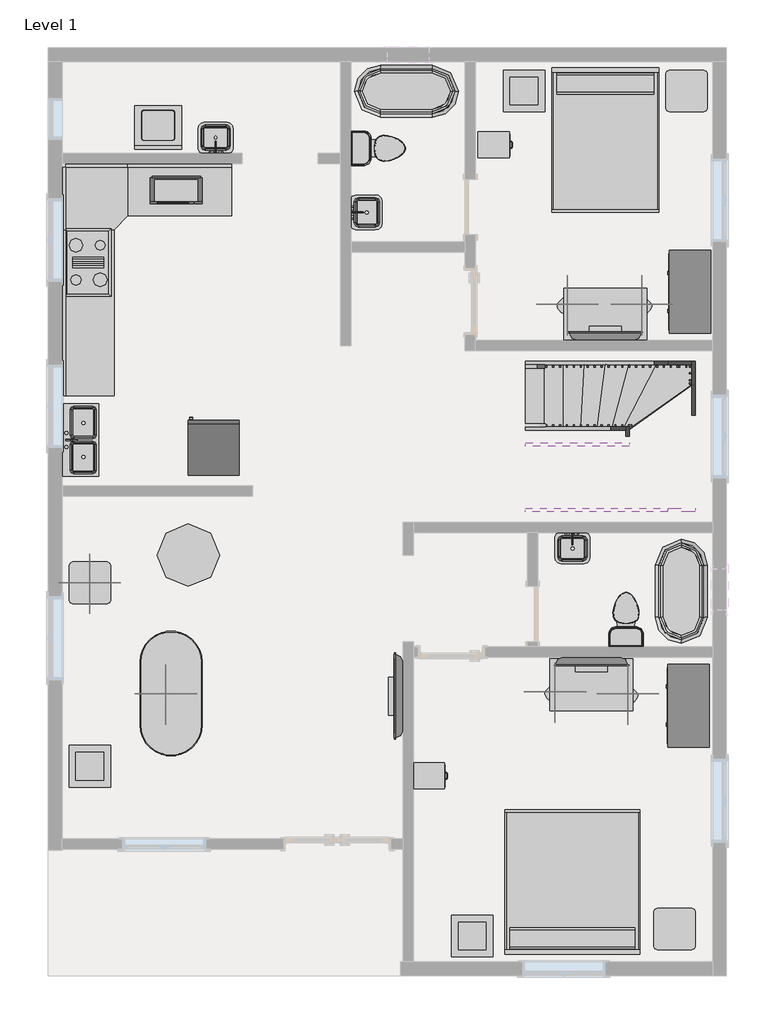
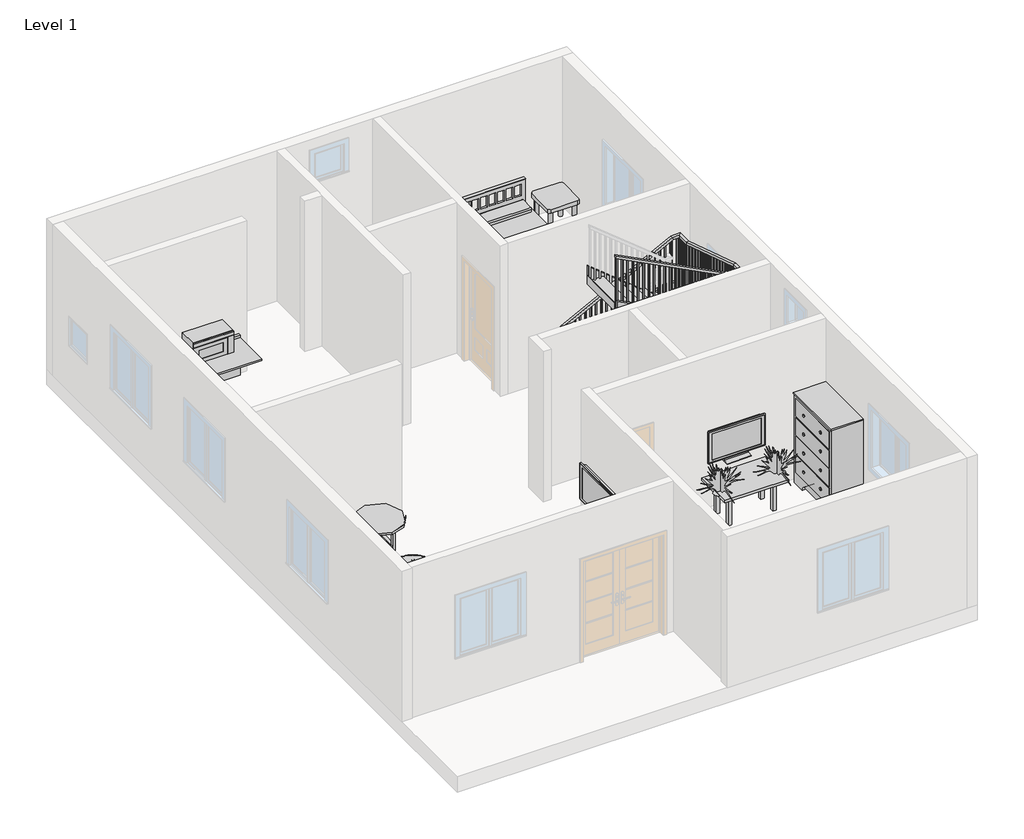
# One storey, part 2 of 2: 20 furniture elements, 11 flow terminals, 8 members, 6 geographic elements, 4 proxies, 1 railing, 1 stair flight.
"""IFC4 building model written with IfcOpenShell, lengths in millimetres."""

from ifc_helpers import new_model, si_unit, frame, origin, place, context, project, spatial, polyline, outline, extrude, faceted_brep, transform, mapped, element, save
from components import proxy_bb1e6e30, proxy_8a8d5ab2, proxy_a13a33b2, proxy_718fa39f, flow_terminal_accce45a, flow_terminal_a53be723, flow_terminal_62a433f7, toilet_domestic_3d_toilet_domestic_3d_f7549cf7, toilet_domestic_3d_toilet_domestic_3d_183bbd19, flow_terminal_b374fae2, furniture_29cd36cd, furniture_35c09872, furniture_bb55ed6b, furniture_9fa109b2, furniture_7a3aaa4f, furniture_fdf74506, furniture_b5c51a22, furniture_2c34a4f9, furniture_905aceb5, furniture_31d08a24, furniture_3f969c1c, furniture_f7403a93, rpc_plant_tropical_agave_1_5_93a2a214, stair_flight_cbf97d32

model = new_model("IFC4")

# Units and contexts
model_context = context("Model", 3, world=origin())
ifc_project = project(units=[si_unit("LENGTHUNIT", "METRE", prefix="MILLI")], contexts=[model_context])

# Site, building, storey
site = spatial("IfcSite", under=ifc_project)
building = spatial("IfcBuilding", under=site)
storey = spatial("IfcBuildingStorey", under=building, Name="Level 1", Elevation=0.0)

# Proxies
placement = place(None, origin())
proxy_shape = proxy_bb1e6e30(model_context)
element("IfcBuildingElementProxy", 1, Name="Cook Top-4 Unit : 36\" x 20\"", ObjectType="Cook Top-4 Unit : 36\" x 20\"", at=placement, inside=storey, context=model_context, shape_type="MappedRepresentation", body=[
    mapped(proxy_shape, transform((-14225.9837964, 8614.5759458, 0.0), x_axis=(0.0, 1.0, 0.0), y_axis=(-1.0, 0.0, 0.0), z_axis=(0.0, 0.0, 1.0))),
])
proxy_2_shape = proxy_8a8d5ab2(model_context)
element("IfcBuildingElementProxy", 2, Name="Microwave : 30\" x 16\" x 18\"", ObjectType="Microwave : 30\" x 16\" x 18\"", at=placement, inside=storey, context=model_context, shape_type="MappedRepresentation", body=[
    mapped(proxy_2_shape, transform((-13430.8766737, 10034.4564516, 0.0), x_axis=(1.0000000000000009, 0.0, 0.0), y_axis=(0.0, 1.0000000000000009, 0.0), z_axis=(0.0, 0.0, 1.0))),
])
proxy_3_shape = proxy_a13a33b2(model_context)
element("IfcBuildingElementProxy", 3, Name="Refrigerator : 30\" x 32\" RH", ObjectType="Refrigerator : 30\" x 32\" RH", at=placement, inside=storey, context=model_context, shape_type="MappedRepresentation", body=[
    mapped(proxy_3_shape, transform((-12379.7212964, 5878.9249173, 0.0), x_axis=(-1.0000000000000004, 0.0, 0.0), y_axis=(0.0, -1.0000000000000004, 0.0), z_axis=(0.0, 0.0, 1.0))),
])
proxy_4_shape = proxy_718fa39f(model_context)
element("IfcBuildingElementProxy", 4, Name="Washer : 27\" x 25\" x 35\"", ObjectType="Washer : 27\" x 25\" x 35\"", at=placement, inside=storey, context=model_context, shape_type="MappedRepresentation", body=[
    mapped(proxy_4_shape, transform((-12776.8663279, 10874.9255106, 0.0), x_axis=(-1.0000000000000004, 0.0, 0.0), y_axis=(0.0, -1.0000000000000004, 0.0), z_axis=(0.0, 0.0, 1.0))),
])

# Flow terminals
flow_terminal_shape = flow_terminal_accce45a(model_context)
element("IfcFlowTerminal", 5, ObjectType="Floor Drain - Round : 5\" Strainer - 2\" Drain", at=placement, inside=storey, context=model_context, shape_type="MappedRepresentation", body=[
    mapped(flow_terminal_shape, transform((-12574.9837964, 11357.7759458, 0.0), x_axis=(1.0, 0.0, 0.0), y_axis=(0.0, 1.0, 0.0), z_axis=(0.0, 0.0, 1.0))),
])
element("IfcFlowTerminal", 6, ObjectType="Floor Drain - Round : 5\" Strainer - 2\" Drain", at=placement, inside=storey, context=model_context, shape_type="MappedRepresentation", body=[
    mapped(flow_terminal_shape, transform((-8841.1837964, 10494.1759458, 0.0), x_axis=(1.0, 0.0, 0.0), y_axis=(0.0, 1.0, 0.0), z_axis=(0.0, 0.0, 1.0))),
])
element("IfcFlowTerminal", 7, ObjectType="Floor Drain - Round : 5\" Strainer - 2\" Drain", at=placement, inside=storey, context=model_context, shape_type="MappedRepresentation", body=[
    mapped(flow_terminal_shape, transform((-6148.7837964, 4372.7759458, 0.0), x_axis=(1.0, 0.0, 0.0), y_axis=(0.0, 1.0, 0.0), z_axis=(0.0, 0.0, 1.0))),
])
flow_terminal_2_shape = flow_terminal_a53be723(model_context)
element("IfcFlowTerminal", 8, ObjectType="Sink Kitchen-Double : 42\" x 21\"", at=placement, inside=storey, context=model_context, shape_type="MappedRepresentation", body=[
    mapped(flow_terminal_2_shape, transform((-14331.5883953, 5995.3867052, 0.0), x_axis=(0.0, 1.0000000000000002, 0.0), y_axis=(-1.0000000000000002, 0.0, 0.0), z_axis=(0.0, 0.0, 1.0))),
])
flow_terminal_3_shape = flow_terminal_62a433f7(model_context)
element("IfcFlowTerminal", 9, ObjectType="Sink Vanity-Square : 20\" x 18\"", at=placement, inside=storey, context=model_context, shape_type="MappedRepresentation", body=[
    mapped(flow_terminal_3_shape, transform((-12337.0445558, 10394.9213469, 0.0), x_axis=(-1.0000000000000002, 0.0, 0.0), y_axis=(0.0, -1.0000000000000002, 0.0), z_axis=(0.0, 0.0, 1.0))),
])
element("IfcFlowTerminal", 10, ObjectType="Sink Vanity-Square : 20\" x 18\"", at=placement, inside=storey, context=model_context, shape_type="MappedRepresentation", body=[
    mapped(flow_terminal_3_shape, transform((-10185.0383953, 9335.4867052, 0.0), x_axis=(0.0, 1.0000000000000002, 0.0), y_axis=(-1.0000000000000002, 0.0, 0.0), z_axis=(0.0, 0.0, 1.0))),
])
element("IfcFlowTerminal", 11, ObjectType="Sink Vanity-Square : 20\" x 18\"", at=placement, inside=storey, context=model_context, shape_type="MappedRepresentation", body=[
    mapped(flow_terminal_3_shape, transform((-7129.6730369, 4472.0305447, 0.0), x_axis=(1.0, 0.0, 0.0), y_axis=(0.0, 1.0, 0.0), z_axis=(0.0, 0.0, 1.0))),
])
toilet_domestic_3d_toilet_domestic_3d_shape = toilet_domestic_3d_toilet_domestic_3d_f7549cf7(model_context)
toilet_domestic_3d_toilet_domestic_3d_2_shape = toilet_domestic_3d_toilet_domestic_3d_183bbd19(model_context)
element("IfcFlowTerminal", 12, ObjectType="Toilet-Domestic-3D : Toilet-Domestic-3D", at=placement, inside=storey, context=model_context, shape_type="MappedRepresentation", body=[
    mapped(toilet_domestic_3d_toilet_domestic_3d_shape, transform((-9870.487769, 10290.9759458, 0.0), x_axis=(0.0, 1.0000000000000002, 0.0), y_axis=(-1.0000000000000002, 0.0, 0.0), z_axis=(0.0, 0.0, 1.0))),
    mapped(toilet_domestic_3d_toilet_domestic_3d_2_shape, transform((-9870.487769, 10290.9759458, 0.0), x_axis=(0.0, 1.0000000000000002, 0.0), y_axis=(-1.0000000000000002, 0.0, 0.0), z_axis=(0.0, 0.0, 1.0))),
])
element("IfcFlowTerminal", 13, ObjectType="Toilet-Domestic-3D : Toilet-Domestic-3D", at=placement, inside=storey, context=model_context, shape_type="MappedRepresentation", body=[
    mapped(toilet_domestic_3d_toilet_domestic_3d_shape, transform((-6326.5837964, 3470.4719732, 0.0), x_axis=(-1.0000000000000004, 0.0, 0.0), y_axis=(0.0, -1.0000000000000004, 0.0), z_axis=(0.0, 0.0, 1.0))),
    mapped(toilet_domestic_3d_toilet_domestic_3d_2_shape, transform((-6326.5837964, 3470.4719732, 0.0), x_axis=(-1.0000000000000004, 0.0, 0.0), y_axis=(0.0, -1.0000000000000004, 0.0), z_axis=(0.0, 0.0, 1.0))),
])
flow_terminal_4_shape = flow_terminal_b374fae2(model_context)
element("IfcFlowTerminal", 14, ObjectType="Tub-Free Standing-3D : 30\" x 60\"", at=placement, inside=storey, context=model_context, shape_type="MappedRepresentation", body=[
    mapped(flow_terminal_4_shape, transform((-9552.3837964, 11129.1759458, 0.0), x_axis=(0.0, 1.0000000000000002, 0.0), y_axis=(-1.0000000000000002, 0.0, 0.0), z_axis=(0.0, 0.0, 1.0))),
])
element("IfcFlowTerminal", 15, ObjectType="Tub-Free Standing-3D : 30\" x 60\"", at=placement, inside=storey, context=model_context, shape_type="MappedRepresentation", body=[
    mapped(flow_terminal_4_shape, transform((-5513.7837964, 3788.5759458, 0.0), x_axis=(1.0, 0.0, 0.0), y_axis=(0.0, 1.0, 0.0), z_axis=(0.0, 0.0, 1.0))),
])

# Furniture
furniture_shape = furniture_29cd36cd(model_context)
element("IfcFurniture", 16, ObjectType="Bed-Shaker : King 78\" x 83\"", at=placement, inside=storey, context=model_context, shape_type="MappedRepresentation", body=[
    mapped(furniture_shape, transform((-7133.0337964, -1520.0240542, 0.0), x_axis=(-1.0000000000000002, 0.0, 0.0), y_axis=(0.0, -1.0000000000000002, 0.0), z_axis=(0.0, 0.0, 1.0))),
])
furniture_2_shape = furniture_35c09872(model_context)
element("IfcFurniture", 17, ObjectType="Bed-Shaker : Queen 62\" x 83\"", at=placement, inside=storey, context=model_context, shape_type="MappedRepresentation", body=[
    mapped(furniture_2_shape, transform((-6612.3337964, 11459.3759458, 0.0), x_axis=(1.0, 0.0, 0.0), y_axis=(0.0, 1.0, 0.0), z_axis=(0.0, 0.0, 1.0))),
])
furniture_3_shape = furniture_bb55ed6b(model_context)
element("IfcFurniture", 18, ObjectType="Cabinet-File 2 Drawer : 15\" x 18\"", at=placement, inside=storey, context=model_context, shape_type="MappedRepresentation", body=[
    mapped(furniture_3_shape, transform((-8411.8180965, 10469.6723928, 0.0), x_axis=(0.0, 1.0000000000000002, 0.0), y_axis=(-1.0000000000000002, 0.0, 0.0), z_axis=(0.0, 0.0, 1.0))),
])
element("IfcFurniture", 19, ObjectType="Cabinet-File 2 Drawer : 15\" x 18\"", at=placement, inside=storey, context=model_context, shape_type="MappedRepresentation", body=[
    mapped(furniture_3_shape, transform((-9364.3180965, 1211.3723928, 0.0), x_axis=(0.0, 1.0, 0.0), y_axis=(-1.0, 0.0, 0.0), z_axis=(0.0, 0.0, 1.0))),
])
furniture_4_shape = furniture_9fa109b2(model_context)
element("IfcFurniture", 20, ObjectType="Dresser : 48\" x 72\" x 24\"", at=placement, inside=storey, context=model_context, shape_type="MappedRepresentation", body=[
    mapped(furniture_4_shape, transform((-5023.6208423, 7913.582686, 0.0), x_axis=(0.0, -1.0000000000000007, 0.0), y_axis=(1.0000000000000007, 0.0, 0.0), z_axis=(0.0, 0.0, 1.0))),
])
element("IfcFurniture", 21, ObjectType="Dresser : 48\" x 72\" x 24\"", at=placement, inside=storey, context=model_context, shape_type="MappedRepresentation", body=[
    mapped(furniture_4_shape, transform((-5049.0208423, 1842.982686, 0.0), x_axis=(0.0, -1.0000000000000004, 0.0), y_axis=(1.0000000000000004, 0.0, 0.0), z_axis=(0.0, 0.0, 1.0))),
])
furniture_5_shape = furniture_7a3aaa4f(model_context)
element("IfcFurniture", 22, ObjectType="TV - Flat Screen : 42\"", at=placement, inside=storey, context=model_context, shape_type="MappedRepresentation", body=[
    mapped(furniture_5_shape, transform((-6635.3283105, 7530.1145695, 914.4), x_axis=(-1.0000000000000004, 0.0, 0.0), y_axis=(0.0, -1.0000000000000004, 0.0), z_axis=(0.0, 0.0, 1.0))),
])
element("IfcFurniture", 23, ObjectType="TV - Flat Screen : 42\"", at=placement, inside=storey, context=model_context, shape_type="MappedRepresentation", body=[
    mapped(furniture_5_shape, transform((-6830.6392822, 2764.8373222, 914.4), x_axis=(1.0, 0.0, 0.0), y_axis=(0.0, 1.0, 0.0), z_axis=(0.0, 0.0, 1.0))),
])
furniture_6_shape = furniture_fdf74506(model_context)
element("IfcFurniture", 24, ObjectType="TV - Flat Screen : 50\"", at=placement, inside=storey, context=model_context, shape_type="MappedRepresentation", body=[
    mapped(furniture_6_shape, transform((-9661.72242, 2247.9314317, 914.4), x_axis=(0.0, -1.0000000000000002, 0.0), y_axis=(1.0000000000000002, 0.0, 0.0), z_axis=(0.0, 0.0, 1.0))),
])
furniture_7_shape = furniture_b5c51a22(model_context)
element("IfcFurniture", 25, ObjectType="Table-Coffee : 24\" x 24\" x 24\"", at=placement, inside=storey, context=model_context, shape_type="MappedRepresentation", body=[
    mapped(furniture_7_shape, transform((-7843.449563, 11033.964868, 0.0), x_axis=(1.0, 0.0, 0.0), y_axis=(0.0, 1.0, 0.0), z_axis=(0.0, 0.0, 1.0))),
])
element("IfcFurniture", 26, ObjectType="Table-Coffee : 24\" x 24\" x 24\"", at=placement, inside=storey, context=model_context, shape_type="MappedRepresentation", body=[
    mapped(furniture_7_shape, transform((-8605.449563, -1361.235132, 0.0), x_axis=(1.0, 0.0, 0.0), y_axis=(0.0, 1.0, 0.0), z_axis=(0.0, 0.0, 1.0))),
])
element("IfcFurniture", 27, ObjectType="Table-Coffee : 24\" x 24\" x 24\"", at=placement, inside=storey, context=model_context, shape_type="MappedRepresentation", body=[
    mapped(furniture_7_shape, transform((-14218.849563, 1127.964868, 0.0), x_axis=(1.0, 0.0, 0.0), y_axis=(0.0, 1.0, 0.0), z_axis=(0.0, 0.0, 1.0))),
])
furniture_8_shape = furniture_2c34a4f9(model_context)
element("IfcFurniture", 28, ObjectType="Table-Dining Oval : 36\" x 72\"", at=placement, inside=storey, context=model_context, shape_type="MappedRepresentation", body=[
    mapped(furniture_8_shape, transform((-13364.882157, 2691.7956179, 0.0), x_axis=(0.0, 1.0, 0.0), y_axis=(-1.0, 0.0, 0.0), z_axis=(0.0, 0.0, 1.0))),
])
furniture_9_shape = furniture_905aceb5(model_context)
element("IfcFurniture", 29, ObjectType="Table-Dining Round w Chairs : 36\" Diameter", at=placement, inside=storey, context=model_context, shape_type="MappedRepresentation", body=[
    mapped(furniture_9_shape, transform((-12856.4657636, 4506.8546343, 0.0), x_axis=(1.0, 0.0, 0.0), y_axis=(0.0, 1.0, 0.0), z_axis=(0.0, 0.0, 1.0))),
])
furniture_10_shape = furniture_31d08a24(model_context)
element("IfcFurniture", 30, ObjectType="Table-End : 24\" x 24\"", at=placement, inside=storey, context=model_context, shape_type="MappedRepresentation", body=[
    mapped(furniture_10_shape, transform((-5746.1174267, 10976.7759458, 0.0), x_axis=(1.0, 0.0, 0.0), y_axis=(0.0, 1.0, 0.0), z_axis=(0.0, 0.0, 1.0))),
])
element("IfcFurniture", 31, ObjectType="Table-End : 24\" x 24\"", at=placement, inside=storey, context=model_context, shape_type="MappedRepresentation", body=[
    mapped(furniture_10_shape, transform((-5923.9174267, -1316.8240542, 0.0), x_axis=(1.0, 0.0, 0.0), y_axis=(0.0, 1.0, 0.0), z_axis=(0.0, 0.0, 1.0))),
])
element("IfcFurniture", 32, ObjectType="Table-End : 24\" x 24\"", at=placement, inside=storey, context=model_context, shape_type="MappedRepresentation", body=[
    mapped(furniture_10_shape, transform((-14509.1174267, 3763.1759458, 0.0), x_axis=(1.0, 0.0, 0.0), y_axis=(0.0, 1.0, 0.0), z_axis=(0.0, 0.0, 1.0))),
])
furniture_11_shape = furniture_3f969c1c(model_context)
element("IfcFurniture", 33, ObjectType="Table-Rectangular : 72\" x 30\"", at=placement, inside=storey, context=model_context, shape_type="MappedRepresentation", body=[
    mapped(furniture_11_shape, transform((-6834.5837964, 2416.9759458, 0.0), x_axis=(1.0, 0.0, 0.0), y_axis=(0.0, 1.0, 0.0), z_axis=(0.0, 0.0, 1.0))),
])
element("IfcFurniture", 34, ObjectType="Table-Rectangular : 72\" x 30\"", at=placement, inside=storey, context=model_context, shape_type="MappedRepresentation", body=[
    mapped(furniture_11_shape, transform((-6631.3837964, 7852.5759458, 0.0), x_axis=(1.0, 0.0, 0.0), y_axis=(0.0, 1.0, 0.0), z_axis=(0.0, 0.0, 1.0))),
])
furniture_12_shape = furniture_f7403a93(model_context)
element("IfcFurniture", 35, ObjectType="Work Station Cubicle : 96\" x 96\"", at=placement, inside=storey, context=model_context, shape_type="MappedRepresentation", body=[
    mapped(furniture_12_shape, transform((-14475.2520442, 10557.3989534, 0.0), x_axis=(1.0, 0.0, 0.0), y_axis=(0.0, 1.0, 0.0), z_axis=(0.0, 0.0, 1.0))),
])

# Geographic elements
rpc_plant_tropical_agave_1_5_shape = rpc_plant_tropical_agave_1_5_93a2a214(model_context)
element("IfcGeographicElement", 36, ObjectType="RPC Plant - Tropical : Agave - 1.5'", at=placement, inside=storey, context=model_context, shape_type="MappedRepresentation", body=[
    mapped(rpc_plant_tropical_agave_1_5_shape, transform((-14200.5837964, 3915.5759458, 609.6), x_axis=(1.0, 0.0, 0.0), y_axis=(0.0, 1.0, 0.0), z_axis=(0.0, 0.0, 1.0))),
])
element("IfcGeographicElement", 37, ObjectType="RPC Plant - Tropical : Agave - 1.5'", at=placement, inside=storey, context=model_context, shape_type="MappedRepresentation", body=[
    mapped(rpc_plant_tropical_agave_1_5_shape, transform((-13082.9837964, 2289.9759458, 736.6), x_axis=(1.0, 0.0, 0.0), y_axis=(0.0, 1.0, 0.0), z_axis=(0.0, 0.0, 1.0))),
])
element("IfcGeographicElement", 38, ObjectType="RPC Plant - Tropical : Agave - 1.5'", at=placement, inside=storey, context=model_context, shape_type="MappedRepresentation", body=[
    mapped(rpc_plant_tropical_agave_1_5_shape, transform((-7367.9837964, 2315.3759458, 660.4), x_axis=(1.0, 0.0, 0.0), y_axis=(0.0, 1.0, 0.0), z_axis=(0.0, 0.0, 1.0))),
])
element("IfcGeographicElement", 39, ObjectType="RPC Plant - Tropical : Agave - 1.5'", at=placement, inside=storey, context=model_context, shape_type="MappedRepresentation", body=[
    mapped(rpc_plant_tropical_agave_1_5_shape, transform((-6301.1837964, 2289.9759458, 660.4), x_axis=(1.0, 0.0, 0.0), y_axis=(0.0, 1.0, 0.0), z_axis=(0.0, 0.0, 1.0))),
])
element("IfcGeographicElement", 40, ObjectType="RPC Plant - Tropical : Agave - 1.5'", at=placement, inside=storey, context=model_context, shape_type="MappedRepresentation", body=[
    mapped(rpc_plant_tropical_agave_1_5_shape, transform((-7190.1837964, 8004.9759458, 660.4), x_axis=(1.0, 0.0, 0.0), y_axis=(0.0, 1.0, 0.0), z_axis=(0.0, 0.0, 1.0))),
])
element("IfcGeographicElement", 41, ObjectType="RPC Plant - Tropical : Agave - 1.5'", at=placement, inside=storey, context=model_context, shape_type="MappedRepresentation", body=[
    mapped(rpc_plant_tropical_agave_1_5_shape, transform((-6097.9837964, 8004.9759458, 660.4), x_axis=(1.0, 0.0, 0.0), y_axis=(0.0, 1.0, 0.0), z_axis=(0.0, 0.0, 1.0))),
])

# Members
element("IfcMember", 42, ObjectType="Stringer - 2\" Width", at=placement, inside=storey, context=model_context, shape_type="SweptSolid", body=[
    extrude(outline(polyline([(229.639954, -7803.5154882), (0.0, -7803.5154882), (0.0, -7583.7531707), (962.500629, -5716.0982966), (1305.3956453, -5716.0982966), (229.639954, -7803.5154882)])), frame((0.0, 7115.9759458, 0.0), z_axis=(0.0, 1.0, 0.0), x_axis=(0.0, 0.0, 1.0)), (0.0, 0.0, 1.0), 50.8),
])
element("IfcMember", 43, ObjectType="Stringer - 2\" Width", at=placement, inside=storey, context=model_context, shape_type="SweptSolid", body=[
    extrude(outline(polyline([(-5716.0982966, 7115.9759458), (-5716.0982966, 7166.7759458), (-5361.3837964, 7166.7759458), (-5361.3837964, 7115.9759458), (-5716.0982966, 7115.9759458)])), frame((0.0, 0.0, 962.500629), z_axis=(0.0, 0.0, 1.0), x_axis=(1.0, 0.0, 0.0)), (0.0, 0.0, 1.0), 342.8950162),
])
element("IfcMember", 44, ObjectType="Stringer - 2\" Width", at=placement, inside=storey, context=model_context, shape_type="SweptSolid", body=[
    extrude(outline(polyline([(7166.7759458, 1289.0952212), (7166.7759458, 1000.5956453), (6997.2534628, 1000.5956453), (5007.7759458, 1638.9682298), (5007.7759458, 1969.9972697), (5044.7560631, 1969.9972697), (7166.7759458, 1289.0952212)])), frame((-5361.3837964, 0.0, 0.0), z_axis=(1.0, 0.0, 0.0), x_axis=(0.0, 1.0, 0.0)), (0.0, 0.0, 1.0), 50.8),
])
element("IfcMember", 45, ObjectType="Stringer - 2\" Width", at=placement, inside=storey, context=model_context, shape_type="SweptSolid", body=[
    extrude(outline(polyline([(-5310.5837964, 5007.7759458), (-5310.5837964, 4956.9759458), (-5716.0982966, 4956.9759458), (-5716.0982966, 5007.7759458), (-5310.5837964, 5007.7759458)])), frame((0.0, 0.0, 1649.8904473), z_axis=(0.0, 0.0, 1.0), x_axis=(1.0, 0.0, 0.0)), (0.0, 0.0, 1.0), 320.1068224),
])
element("IfcMember", 46, ObjectType="Stringer - 2\" Width", at=placement, inside=storey, context=model_context, shape_type="SweptSolid", body=[
    extrude(outline(polyline([(1649.8904473, -5716.0982966), (1969.9972697, -5716.0982966), (3045.7529609, -7803.5154882), (2725.6461385, -7803.5154882), (1649.8904473, -5716.0982966)])), frame((0.0, 4956.9759458, 0.0), z_axis=(0.0, 1.0, 0.0), x_axis=(0.0, 0.0, 1.0)), (0.0, 0.0, 1.0), 50.8),
])
element("IfcMember", 47, ObjectType="Stringer - 2\" Width", at=placement, inside=storey, context=model_context, shape_type="SweptSolid", body=[
    extrude(outline(polyline([(176.1764461, -7803.5154882), (0.0, -7803.5154882), (0.0, -7537.2538437), (987.1410923, -6326.5837964), (1380.418648, -6326.5837964), (176.1764461, -7803.5154882)])), frame((0.0, 6150.7759458, 0.0), z_axis=(0.0, 1.0, 0.0), x_axis=(0.0, 0.0, 1.0)), (0.0, 0.0, 1.0), 50.8),
])
element("IfcMember", 48, ObjectType="Stringer - 2\" Width", at=placement, inside=storey, context=model_context, shape_type="SweptSolid", body=[
    extrude(outline(polyline([(6201.5759458, 1573.2682978), (6201.5759458, 1028.5617647), (6167.3337285, 1028.5617647), (5972.9759458, 1360.465107), (5972.9759458, 1926.1409689), (5994.9388284, 1926.1409689), (6201.5759458, 1573.2682978)])), frame((-6326.5837964, 0.0, 0.0), z_axis=(1.0, 0.0, 0.0), x_axis=(0.0, 1.0, 0.0)), (0.0, 0.0, 1.0), 50.8),
])
element("IfcMember", 49, ObjectType="Stringer - 2\" Width", at=placement, inside=storey, context=model_context, shape_type="SweptSolid", body=[
    extrude(outline(polyline([(1532.8634131, -6275.7837964), (1926.1409689, -6275.7837964), (3171.8038432, -7803.5154882), (2778.5262875, -7803.5154882), (1532.8634131, -6275.7837964)])), frame((0.0, 5922.1759458, 0.0), z_axis=(0.0, 1.0, 0.0), x_axis=(0.0, 0.0, 1.0)), (0.0, 0.0, 1.0), 50.8),
])

# Railing
element("IfcRailing", 50, ObjectType="Handrail - Rectangular", at=placement, inside=storey, context=model_context, shape_type="SolidModel", body=[
    faceted_brep([(-7803.5154882, 7115.9759458, 1109.0771751), (-7803.5154882, 7115.9759458, 1051.9280057), (-7803.5154882, 7065.1759458, 1051.9280057), (-7803.5154882, 7065.1759458, 1109.0771751), (-5543.5336317, 7115.9759458, 2273.7644996), (-5531.2135805, 7115.9759458, 2222.9644996), (-5531.2135805, 7065.1759458, 2222.9644996), (-5543.5336317, 7065.1759458, 2273.7644996), (-5361.3837964, 7115.9759458, 2273.7644996), (-5361.3837964, 7115.9759458, 2222.9644996), (-5412.1837964, 7065.1759458, 2222.9644996), (-5412.1837964, 7065.1759458, 2273.7644996), (-5361.3837964, 6838.8219932, 2273.7644996), (-5361.3837964, 6830.8714171, 2222.9644996), (-5412.1837964, 6830.8714171, 2222.9644996), (-5412.1837964, 6838.8219932, 2273.7644996), (-5361.3837964, 5284.9298984, 2772.3688337), (-5361.3837964, 5276.9793223, 2721.5688337), (-5412.1837964, 5276.9793223, 2721.5688337), (-5412.1837964, 5284.9298984, 2772.3688337), (-5361.3837964, 5007.7759458, 2772.3688337), (-5361.3837964, 5007.7759458, 2721.5688337), (-5412.1837964, 5058.5759458, 2721.5688337), (-5412.1837964, 5058.5759458, 2772.3688337), (-5543.5336317, 5007.7759458, 2772.3688337), (-5555.853683, 5007.7759458, 2721.5688337), (-5555.853683, 5058.5759458, 2721.5688337), (-5543.5336317, 5058.5759458, 2772.3688337), (-7803.5154882, 5007.7759458, 3937.0561582), (-7803.5154882, 5058.5759458, 3937.0561582), (-7803.5154882, 5058.5759458, 3879.9069889), (-7803.5154882, 5007.7759458, 3879.9069889)], [[[0, 1, 2, 3]], [[1, 0, 4, 5]], [[2, 1, 5, 6]], [[3, 2, 6, 7]], [[0, 3, 7, 4]], [[5, 4, 8, 9]], [[6, 5, 9, 10]], [[7, 6, 10, 11]], [[4, 7, 11, 8]], [[9, 8, 12, 13]], [[10, 9, 13, 14]], [[11, 10, 14, 15]], [[8, 11, 15, 12]], [[13, 12, 16, 17]], [[14, 13, 17, 18]], [[15, 14, 18, 19]], [[12, 15, 19, 16]], [[17, 16, 20, 21]], [[18, 17, 21, 22]], [[19, 18, 22, 23]], [[16, 19, 23, 20]], [[21, 20, 24, 25]], [[22, 21, 25, 26]], [[23, 22, 26, 27]], [[20, 23, 27, 24]], [[28, 29, 30, 31]], [[25, 24, 28, 31]], [[26, 25, 31, 30]], [[27, 26, 30, 29]], [[24, 27, 29, 28]]]),
    extrude(outline(polyline([(3872.0443296, -7788.2586317), (2878.6666667, -7788.2586317), (2878.6666667, -7769.2086317), (3862.2268642, -7769.2086317), (3872.0443296, -7788.2586317)])), frame((0.0, 5023.6509458, 0.0), z_axis=(0.0, 1.0, 0.0), x_axis=(0.0, 0.0, 1.0)), (0.0, 0.0, 1.0), 19.05),
    extrude(outline(polyline([(3819.6845145, -7686.6586317), (2878.6666667, -7686.6586317), (2878.6666667, -7667.6086317), (3809.8670491, -7667.6086317), (3819.6845145, -7686.6586317)])), frame((0.0, 5023.6509458, 0.0), z_axis=(0.0, 1.0, 0.0), x_axis=(0.0, 0.0, 1.0)), (0.0, 0.0, 1.0), 19.05),
    extrude(outline(polyline([(3767.3246993, -7585.0586317), (2878.6666667, -7585.0586317), (2878.6666667, -7566.0086317), (3757.507234, -7566.0086317), (3767.3246993, -7585.0586317)])), frame((0.0, 5023.6509458, 0.0), z_axis=(0.0, 1.0, 0.0), x_axis=(0.0, 0.0, 1.0)), (0.0, 0.0, 1.0), 19.05),
    extrude(outline(polyline([(3714.9648842, -7483.4586317), (2709.3333333, -7483.4586317), (2709.3333333, -7464.4086317), (3705.1474189, -7464.4086317), (3714.9648842, -7483.4586317)])), frame((0.0, 5023.6509458, 0.0), z_axis=(0.0, 1.0, 0.0), x_axis=(0.0, 0.0, 1.0)), (0.0, 0.0, 1.0), 19.05),
    extrude(outline(polyline([(3662.6050691, -7381.8586317), (2709.3333333, -7381.8586317), (2709.3333333, -7362.8086317), (3652.7876038, -7362.8086317), (3662.6050691, -7381.8586317)])), frame((0.0, 5023.6509458, 0.0), z_axis=(0.0, 1.0, 0.0), x_axis=(0.0, 0.0, 1.0)), (0.0, 0.0, 1.0), 19.05),
    extrude(outline(polyline([(3610.245254, -7280.2586317), (2709.3333333, -7280.2586317), (2709.3333333, -7261.2086317), (3600.4277887, -7261.2086317), (3610.245254, -7280.2586317)])), frame((0.0, 5023.6509458, 0.0), z_axis=(0.0, 1.0, 0.0), x_axis=(0.0, 0.0, 1.0)), (0.0, 0.0, 1.0), 19.05),
    extrude(outline(polyline([(3557.8854389, -7178.6586317), (2540.0, -7178.6586317), (2540.0, -7159.6086317), (3548.0679735, -7159.6086317), (3557.8854389, -7178.6586317)])), frame((0.0, 5023.6509458, 0.0), z_axis=(0.0, 1.0, 0.0), x_axis=(0.0, 0.0, 1.0)), (0.0, 0.0, 1.0), 19.05),
    extrude(outline(polyline([(3505.5256238, -7077.0586317), (2540.0, -7077.0586317), (2540.0, -7058.0086317), (3495.7081584, -7058.0086317), (3505.5256238, -7077.0586317)])), frame((0.0, 5023.6509458, 0.0), z_axis=(0.0, 1.0, 0.0), x_axis=(0.0, 0.0, 1.0)), (0.0, 0.0, 1.0), 19.05),
    extrude(outline(polyline([(3453.1658086, -6975.4586317), (2540.0, -6975.4586317), (2540.0, -6956.4086317), (3443.3483433, -6956.4086317), (3453.1658086, -6975.4586317)])), frame((0.0, 5023.6509458, 0.0), z_axis=(0.0, 1.0, 0.0), x_axis=(0.0, 0.0, 1.0)), (0.0, 0.0, 1.0), 19.05),
    extrude(outline(polyline([(3400.8059935, -6873.8586317), (2370.6666667, -6873.8586317), (2370.6666667, -6854.8086317), (3390.9885282, -6854.8086317), (3400.8059935, -6873.8586317)])), frame((0.0, 5023.6509458, 0.0), z_axis=(0.0, 1.0, 0.0), x_axis=(0.0, 0.0, 1.0)), (0.0, 0.0, 1.0), 19.05),
    extrude(outline(polyline([(3348.4461784, -6772.2586317), (2370.6666667, -6772.2586317), (2370.6666667, -6753.2086317), (3338.6287131, -6753.2086317), (3348.4461784, -6772.2586317)])), frame((0.0, 5023.6509458, 0.0), z_axis=(0.0, 1.0, 0.0), x_axis=(0.0, 0.0, 1.0)), (0.0, 0.0, 1.0), 19.05),
    extrude(outline(polyline([(3296.0863633, -6670.6586317), (2370.6666667, -6670.6586317), (2370.6666667, -6651.6086317), (3286.268898, -6651.6086317), (3296.0863633, -6670.6586317)])), frame((0.0, 5023.6509458, 0.0), z_axis=(0.0, 1.0, 0.0), x_axis=(0.0, 0.0, 1.0)), (0.0, 0.0, 1.0), 19.05),
    extrude(outline(polyline([(3243.7265482, -6569.0586317), (2201.3333333, -6569.0586317), (2201.3333333, -6550.0086317), (3233.9090828, -6550.0086317), (3243.7265482, -6569.0586317)])), frame((0.0, 5023.6509458, 0.0), z_axis=(0.0, 1.0, 0.0), x_axis=(0.0, 0.0, 1.0)), (0.0, 0.0, 1.0), 19.05),
    extrude(outline(polyline([(3191.3667331, -6467.4586317), (2201.3333333, -6467.4586317), (2201.3333333, -6448.4086317), (3181.5492677, -6448.4086317), (3191.3667331, -6467.4586317)])), frame((0.0, 5023.6509458, 0.0), z_axis=(0.0, 1.0, 0.0), x_axis=(0.0, 0.0, 1.0)), (0.0, 0.0, 1.0), 19.05),
    extrude(outline(polyline([(3139.0069179, -6365.8586317), (2201.3333333, -6365.8586317), (2201.3333333, -6346.8086317), (3129.1894526, -6346.8086317), (3139.0069179, -6365.8586317)])), frame((0.0, 5023.6509458, 0.0), z_axis=(0.0, 1.0, 0.0), x_axis=(0.0, 0.0, 1.0)), (0.0, 0.0, 1.0), 19.05),
    extrude(outline(polyline([(3086.6471028, -6264.2586317), (2032.0, -6264.2586317), (2032.0, -6245.2086317), (3076.8296375, -6245.2086317), (3086.6471028, -6264.2586317)])), frame((0.0, 5023.6509458, 0.0), z_axis=(0.0, 1.0, 0.0), x_axis=(0.0, 0.0, 1.0)), (0.0, 0.0, 1.0), 19.05),
    extrude(outline(polyline([(3034.2872877, -6162.6586317), (2032.0, -6162.6586317), (2032.0, -6143.6086317), (3024.4698224, -6143.6086317), (3034.2872877, -6162.6586317)])), frame((0.0, 5023.6509458, 0.0), z_axis=(0.0, 1.0, 0.0), x_axis=(0.0, 0.0, 1.0)), (0.0, 0.0, 1.0), 19.05),
    extrude(outline(polyline([(2981.9274726, -6061.0586317), (2032.0, -6061.0586317), (2032.0, -6042.0086317), (2972.1100073, -6042.0086317), (2981.9274726, -6061.0586317)])), frame((0.0, 5023.6509458, 0.0), z_axis=(0.0, 1.0, 0.0), x_axis=(0.0, 0.0, 1.0)), (0.0, 0.0, 1.0), 19.05),
    extrude(outline(polyline([(2929.5676575, -5959.4586317), (2032.0, -5959.4586317), (2032.0, -5940.4086317), (2919.7501921, -5940.4086317), (2929.5676575, -5959.4586317)])), frame((0.0, 5023.6509458, 0.0), z_axis=(0.0, 1.0, 0.0), x_axis=(0.0, 0.0, 1.0)), (0.0, 0.0, 1.0), 19.05),
    extrude(outline(polyline([(2877.2078424, -5857.8586317), (1862.6666667, -5857.8586317), (1862.6666667, -5838.8086317), (2867.390377, -5838.8086317), (2877.2078424, -5857.8586317)])), frame((0.0, 5023.6509458, 0.0), z_axis=(0.0, 1.0, 0.0), x_axis=(0.0, 0.0, 1.0)), (0.0, 0.0, 1.0), 19.05),
    extrude(outline(polyline([(2824.8480272, -5756.2586317), (1862.6666667, -5756.2586317), (1862.6666667, -5737.2086317), (2815.0305619, -5737.2086317), (2824.8480272, -5756.2586317)])), frame((0.0, 5023.6509458, 0.0), z_axis=(0.0, 1.0, 0.0), x_axis=(0.0, 0.0, 1.0)), (0.0, 0.0, 1.0), 19.05),
    extrude(outline(polyline([(2772.4882121, -5654.6586317), (1862.6666667, -5654.6586317), (1862.6666667, -5635.6086317), (2762.6707468, -5635.6086317), (2772.4882121, -5654.6586317)])), frame((0.0, 5023.6509458, 0.0), z_axis=(0.0, 1.0, 0.0), x_axis=(0.0, 0.0, 1.0)), (0.0, 0.0, 1.0), 19.05),
    extrude(outline(polyline([(-5478.8587964, 5023.6509458), (-5497.9087964, 5023.6509458), (-5497.9087964, 5042.7009458), (-5478.8587964, 5042.7009458), (-5478.8587964, 5023.6509458)])), frame((0.0, 0.0, 1862.6666667), z_axis=(0.0, 0.0, 1.0), x_axis=(1.0, 0.0, 0.0)), (0.0, 0.0, 1.0), 858.902167),
    extrude(outline(polyline([(-5377.2587964, 5091.2548984), (-5377.2587964, 5072.2048984), (-5396.3087964, 5072.2048984), (-5396.3087964, 5091.2548984), (-5377.2587964, 5091.2548984)])), frame((0.0, 0.0, 1862.6666667), z_axis=(0.0, 0.0, 1.0), x_axis=(1.0, 0.0, 0.0)), (0.0, 0.0, 1.0), 858.902167),
    extrude(outline(polyline([(-5377.2587964, 5192.8548984), (-5377.2587964, 5173.8048984), (-5396.3087964, 5173.8048984), (-5396.3087964, 5192.8548984), (-5377.2587964, 5192.8548984)])), frame((0.0, 0.0, 1862.6666667), z_axis=(0.0, 0.0, 1.0), x_axis=(1.0, 0.0, 0.0)), (0.0, 0.0, 1.0), 858.902167),
    extrude(outline(polyline([(5324.3469932, 2706.3697564), (5324.3469932, 1693.3333333), (5305.2969932, 1693.3333333), (5305.2969932, 2712.4824155), (5324.3469932, 2706.3697564)])), frame((-5396.3087964, 0.0, 0.0), z_axis=(1.0, 0.0, 0.0), x_axis=(0.0, 1.0, 0.0)), (0.0, 0.0, 1.0), 19.05),
    extrude(outline(polyline([(5425.9469932, 2673.7689082), (5425.9469932, 1693.3333333), (5406.8969932, 1693.3333333), (5406.8969932, 2679.8815673), (5425.9469932, 2673.7689082)])), frame((-5396.3087964, 0.0, 0.0), z_axis=(1.0, 0.0, 0.0), x_axis=(0.0, 1.0, 0.0)), (0.0, 0.0, 1.0), 19.05),
    extrude(outline(polyline([(5527.5469932, 2641.16806), (5527.5469932, 1693.3333333), (5508.4969932, 1693.3333333), (5508.4969932, 2647.280719), (5527.5469932, 2641.16806)])), frame((-5396.3087964, 0.0, 0.0), z_axis=(1.0, 0.0, 0.0), x_axis=(0.0, 1.0, 0.0)), (0.0, 0.0, 1.0), 19.05),
    extrude(outline(polyline([(5629.1469932, 2608.5672118), (5629.1469932, 1693.3333333), (5610.0969932, 1693.3333333), (5610.0969932, 2614.6798708), (5629.1469932, 2608.5672118)])), frame((-5396.3087964, 0.0, 0.0), z_axis=(1.0, 0.0, 0.0), x_axis=(0.0, 1.0, 0.0)), (0.0, 0.0, 1.0), 19.05),
    extrude(outline(polyline([(5730.7469932, 2575.9663635), (5730.7469932, 1693.3333333), (5711.6969932, 1693.3333333), (5711.6969932, 2582.0790226), (5730.7469932, 2575.9663635)])), frame((-5396.3087964, 0.0, 0.0), z_axis=(1.0, 0.0, 0.0), x_axis=(0.0, 1.0, 0.0)), (0.0, 0.0, 1.0), 19.05),
    extrude(outline(polyline([(5832.3469932, 2543.3655153), (5832.3469932, 1693.3333333), (5813.2969932, 1693.3333333), (5813.2969932, 2549.4781744), (5832.3469932, 2543.3655153)])), frame((-5396.3087964, 0.0, 0.0), z_axis=(1.0, 0.0, 0.0), x_axis=(0.0, 1.0, 0.0)), (0.0, 0.0, 1.0), 19.05),
    extrude(outline(polyline([(5933.9469932, 2510.7646671), (5933.9469932, 1524.0), (5914.8969932, 1524.0), (5914.8969932, 2516.8773261), (5933.9469932, 2510.7646671)])), frame((-5396.3087964, 0.0, 0.0), z_axis=(1.0, 0.0, 0.0), x_axis=(0.0, 1.0, 0.0)), (0.0, 0.0, 1.0), 19.05),
    extrude(outline(polyline([(6035.5469932, 2478.1638189), (6035.5469932, 1524.0), (6016.4969932, 1524.0), (6016.4969932, 2484.2764779), (6035.5469932, 2478.1638189)])), frame((-5396.3087964, 0.0, 0.0), z_axis=(1.0, 0.0, 0.0), x_axis=(0.0, 1.0, 0.0)), (0.0, 0.0, 1.0), 19.05),
    extrude(outline(polyline([(6137.1469932, 2445.5629706), (6137.1469932, 1524.0), (6118.0969932, 1524.0), (6118.0969932, 2451.6756297), (6137.1469932, 2445.5629706)])), frame((-5396.3087964, 0.0, 0.0), z_axis=(1.0, 0.0, 0.0), x_axis=(0.0, 1.0, 0.0)), (0.0, 0.0, 1.0), 19.05),
    extrude(outline(polyline([(6238.7469932, 2412.9621224), (6238.7469932, 1524.0), (6219.6969932, 1524.0), (6219.6969932, 2419.0747814), (6238.7469932, 2412.9621224)])), frame((-5396.3087964, 0.0, 0.0), z_axis=(1.0, 0.0, 0.0), x_axis=(0.0, 1.0, 0.0)), (0.0, 0.0, 1.0), 19.05),
    extrude(outline(polyline([(6340.3469932, 2380.3612742), (6340.3469932, 1354.6666667), (6321.2969932, 1354.6666667), (6321.2969932, 2386.4739332), (6340.3469932, 2380.3612742)])), frame((-5396.3087964, 0.0, 0.0), z_axis=(1.0, 0.0, 0.0), x_axis=(0.0, 1.0, 0.0)), (0.0, 0.0, 1.0), 19.05),
    extrude(outline(polyline([(6441.9469932, 2347.7604259), (6441.9469932, 1354.6666667), (6422.8969932, 1354.6666667), (6422.8969932, 2353.873085), (6441.9469932, 2347.7604259)])), frame((-5396.3087964, 0.0, 0.0), z_axis=(1.0, 0.0, 0.0), x_axis=(0.0, 1.0, 0.0)), (0.0, 0.0, 1.0), 19.05),
    extrude(outline(polyline([(6543.5469932, 2315.1595777), (6543.5469932, 1354.6666667), (6524.4969932, 1354.6666667), (6524.4969932, 2321.2722368), (6543.5469932, 2315.1595777)])), frame((-5396.3087964, 0.0, 0.0), z_axis=(1.0, 0.0, 0.0), x_axis=(0.0, 1.0, 0.0)), (0.0, 0.0, 1.0), 19.05),
    extrude(outline(polyline([(6645.1469932, 2282.5587295), (6645.1469932, 1354.6666667), (6626.0969932, 1354.6666667), (6626.0969932, 2288.6713885), (6645.1469932, 2282.5587295)])), frame((-5396.3087964, 0.0, 0.0), z_axis=(1.0, 0.0, 0.0), x_axis=(0.0, 1.0, 0.0)), (0.0, 0.0, 1.0), 19.05),
    extrude(outline(polyline([(6746.7469932, 2249.9578813), (6746.7469932, 1354.6666667), (6727.6969932, 1354.6666667), (6727.6969932, 2256.0705403), (6746.7469932, 2249.9578813)])), frame((-5396.3087964, 0.0, 0.0), z_axis=(1.0, 0.0, 0.0), x_axis=(0.0, 1.0, 0.0)), (0.0, 0.0, 1.0), 19.05),
    extrude(outline(polyline([(-5377.2587964, 6896.9009458), (-5377.2587964, 6877.8509458), (-5396.3087964, 6877.8509458), (-5396.3087964, 6896.9009458), (-5377.2587964, 6896.9009458)])), frame((0.0, 0.0, 1185.3333333), z_axis=(0.0, 0.0, 1.0), x_axis=(1.0, 0.0, 0.0)), (0.0, 0.0, 1.0), 1037.6311663),
    extrude(outline(polyline([(-5377.2587964, 6998.5009458), (-5377.2587964, 6979.4509458), (-5396.3087964, 6979.4509458), (-5396.3087964, 6998.5009458), (-5377.2587964, 6998.5009458)])), frame((0.0, 0.0, 1185.3333333), z_axis=(0.0, 0.0, 1.0), x_axis=(1.0, 0.0, 0.0)), (0.0, 0.0, 1.0), 1037.6311663),
    extrude(outline(polyline([(-5451.4586317, 7100.1009458), (-5432.4086317, 7100.1009458), (-5432.4086317, 7081.0509458), (-5451.4586317, 7081.0509458), (-5451.4586317, 7100.1009458)])), frame((0.0, 0.0, 1185.3333333), z_axis=(0.0, 0.0, 1.0), x_axis=(1.0, 0.0, 0.0)), (0.0, 0.0, 1.0), 1037.6311663),
    extrude(outline(polyline([(2198.9352056, -5577.8404882), (1185.3333333, -5577.8404882), (1185.3333333, -5558.7904882), (2208.752671, -5558.7904882), (2198.9352056, -5577.8404882)])), frame((0.0, 7081.0509458, 0.0), z_axis=(0.0, 1.0, 0.0), x_axis=(0.0, 0.0, 1.0)), (0.0, 0.0, 1.0), 19.05),
    extrude(outline(polyline([(2146.5753905, -5679.4404882), (1185.3333333, -5679.4404882), (1185.3333333, -5660.3904882), (2156.3928558, -5660.3904882), (2146.5753905, -5679.4404882)])), frame((0.0, 7081.0509458, 0.0), z_axis=(0.0, 1.0, 0.0), x_axis=(0.0, 0.0, 1.0)), (0.0, 0.0, 1.0), 19.05),
    extrude(outline(polyline([(2094.2155754, -5781.0404882), (1185.3333333, -5781.0404882), (1185.3333333, -5761.9904882), (2104.0330407, -5761.9904882), (2094.2155754, -5781.0404882)])), frame((0.0, 7081.0509458, 0.0), z_axis=(0.0, 1.0, 0.0), x_axis=(0.0, 0.0, 1.0)), (0.0, 0.0, 1.0), 19.05),
    extrude(outline(polyline([(2041.8557603, -5882.6404882), (1185.3333333, -5882.6404882), (1185.3333333, -5863.5904882), (2051.6732256, -5863.5904882), (2041.8557603, -5882.6404882)])), frame((0.0, 7081.0509458, 0.0), z_axis=(0.0, 1.0, 0.0), x_axis=(0.0, 0.0, 1.0)), (0.0, 0.0, 1.0), 19.05),
    extrude(outline(polyline([(1989.4959452, -5984.2404882), (1016.0, -5984.2404882), (1016.0, -5965.1904882), (1999.3134105, -5965.1904882), (1989.4959452, -5984.2404882)])), frame((0.0, 7081.0509458, 0.0), z_axis=(0.0, 1.0, 0.0), x_axis=(0.0, 0.0, 1.0)), (0.0, 0.0, 1.0), 19.05),
    extrude(outline(polyline([(1937.13613, -6085.8404882), (1016.0, -6085.8404882), (1016.0, -6066.7904882), (1946.9535954, -6066.7904882), (1937.13613, -6085.8404882)])), frame((0.0, 7081.0509458, 0.0), z_axis=(0.0, 1.0, 0.0), x_axis=(0.0, 0.0, 1.0)), (0.0, 0.0, 1.0), 19.05),
    extrude(outline(polyline([(1884.7763149, -6187.4404882), (1016.0, -6187.4404882), (1016.0, -6168.3904882), (1894.5937803, -6168.3904882), (1884.7763149, -6187.4404882)])), frame((0.0, 7081.0509458, 0.0), z_axis=(0.0, 1.0, 0.0), x_axis=(0.0, 0.0, 1.0)), (0.0, 0.0, 1.0), 19.05),
    extrude(outline(polyline([(1832.4164998, -6289.0404882), (1016.0, -6289.0404882), (1016.0, -6269.9904882), (1842.2339651, -6269.9904882), (1832.4164998, -6289.0404882)])), frame((0.0, 7081.0509458, 0.0), z_axis=(0.0, 1.0, 0.0), x_axis=(0.0, 0.0, 1.0)), (0.0, 0.0, 1.0), 19.05),
    extrude(outline(polyline([(1780.0566847, -6390.6404882), (846.6666667, -6390.6404882), (846.6666667, -6371.5904882), (1789.87415, -6371.5904882), (1780.0566847, -6390.6404882)])), frame((0.0, 7081.0509458, 0.0), z_axis=(0.0, 1.0, 0.0), x_axis=(0.0, 0.0, 1.0)), (0.0, 0.0, 1.0), 19.05),
    extrude(outline(polyline([(1727.6968696, -6492.2404882), (846.6666667, -6492.2404882), (846.6666667, -6473.1904882), (1737.5143349, -6473.1904882), (1727.6968696, -6492.2404882)])), frame((0.0, 7081.0509458, 0.0), z_axis=(0.0, 1.0, 0.0), x_axis=(0.0, 0.0, 1.0)), (0.0, 0.0, 1.0), 19.05),
    extrude(outline(polyline([(1675.3370545, -6593.8404882), (846.6666667, -6593.8404882), (846.6666667, -6574.7904882), (1685.1545198, -6574.7904882), (1675.3370545, -6593.8404882)])), frame((0.0, 7081.0509458, 0.0), z_axis=(0.0, 1.0, 0.0), x_axis=(0.0, 0.0, 1.0)), (0.0, 0.0, 1.0), 19.05),
    extrude(outline(polyline([(1622.9772393, -6695.4404882), (677.3333333, -6695.4404882), (677.3333333, -6676.3904882), (1632.7947047, -6676.3904882), (1622.9772393, -6695.4404882)])), frame((0.0, 7081.0509458, 0.0), z_axis=(0.0, 1.0, 0.0), x_axis=(0.0, 0.0, 1.0)), (0.0, 0.0, 1.0), 19.05),
    extrude(outline(polyline([(1570.6174242, -6797.0404882), (677.3333333, -6797.0404882), (677.3333333, -6777.9904882), (1580.4348896, -6777.9904882), (1570.6174242, -6797.0404882)])), frame((0.0, 7081.0509458, 0.0), z_axis=(0.0, 1.0, 0.0), x_axis=(0.0, 0.0, 1.0)), (0.0, 0.0, 1.0), 19.05),
    extrude(outline(polyline([(1518.2576091, -6898.6404882), (677.3333333, -6898.6404882), (677.3333333, -6879.5904882), (1528.0750744, -6879.5904882), (1518.2576091, -6898.6404882)])), frame((0.0, 7081.0509458, 0.0), z_axis=(0.0, 1.0, 0.0), x_axis=(0.0, 0.0, 1.0)), (0.0, 0.0, 1.0), 19.05),
    extrude(outline(polyline([(1465.897794, -7000.2404882), (508.0, -7000.2404882), (508.0, -6981.1904882), (1475.7152593, -6981.1904882), (1465.897794, -7000.2404882)])), frame((0.0, 7081.0509458, 0.0), z_axis=(0.0, 1.0, 0.0), x_axis=(0.0, 0.0, 1.0)), (0.0, 0.0, 1.0), 19.05),
    extrude(outline(polyline([(1413.5379789, -7101.8404882), (508.0, -7101.8404882), (508.0, -7082.7904882), (1423.3554442, -7082.7904882), (1413.5379789, -7101.8404882)])), frame((0.0, 7081.0509458, 0.0), z_axis=(0.0, 1.0, 0.0), x_axis=(0.0, 0.0, 1.0)), (0.0, 0.0, 1.0), 19.05),
    extrude(outline(polyline([(1361.1781638, -7203.4404882), (508.0, -7203.4404882), (508.0, -7184.3904882), (1370.9956291, -7184.3904882), (1361.1781638, -7203.4404882)])), frame((0.0, 7081.0509458, 0.0), z_axis=(0.0, 1.0, 0.0), x_axis=(0.0, 0.0, 1.0)), (0.0, 0.0, 1.0), 19.05),
    extrude(outline(polyline([(1308.8183486, -7305.0404882), (338.6666667, -7305.0404882), (338.6666667, -7285.9904882), (1318.635814, -7285.9904882), (1308.8183486, -7305.0404882)])), frame((0.0, 7081.0509458, 0.0), z_axis=(0.0, 1.0, 0.0), x_axis=(0.0, 0.0, 1.0)), (0.0, 0.0, 1.0), 19.05),
    extrude(outline(polyline([(1256.4585335, -7406.6404882), (338.6666667, -7406.6404882), (338.6666667, -7387.5904882), (1266.2759989, -7387.5904882), (1256.4585335, -7406.6404882)])), frame((0.0, 7081.0509458, 0.0), z_axis=(0.0, 1.0, 0.0), x_axis=(0.0, 0.0, 1.0)), (0.0, 0.0, 1.0), 19.05),
    extrude(outline(polyline([(1204.0987184, -7508.2404882), (338.6666667, -7508.2404882), (338.6666667, -7489.1904882), (1213.9161837, -7489.1904882), (1204.0987184, -7508.2404882)])), frame((0.0, 7081.0509458, 0.0), z_axis=(0.0, 1.0, 0.0), x_axis=(0.0, 0.0, 1.0)), (0.0, 0.0, 1.0), 19.05),
    extrude(outline(polyline([(1151.7389033, -7609.8404882), (169.3333333, -7609.8404882), (169.3333333, -7590.7904882), (1161.5563686, -7590.7904882), (1151.7389033, -7609.8404882)])), frame((0.0, 7081.0509458, 0.0), z_axis=(0.0, 1.0, 0.0), x_axis=(0.0, 0.0, 1.0)), (0.0, 0.0, 1.0), 19.05),
    extrude(outline(polyline([(1099.3790882, -7711.4404882), (169.3333333, -7711.4404882), (169.3333333, -7692.3904882), (1109.1965535, -7692.3904882), (1099.3790882, -7711.4404882)])), frame((0.0, 7081.0509458, 0.0), z_axis=(0.0, 1.0, 0.0), x_axis=(0.0, 0.0, 1.0)), (0.0, 0.0, 1.0), 19.05),
    extrude(outline(polyline([(-5534.0086317, 5023.6509458), (-5553.0586317, 5023.6509458), (-5553.0586317, 5042.7009458), (-5534.0086317, 5042.7009458), (-5534.0086317, 5023.6509458)])), frame((0.0, 0.0, 1862.6666667), z_axis=(0.0, 0.0, 1.0), x_axis=(1.0, 0.0, 0.0)), (0.0, 0.0, 1.0), 858.902167),
    extrude(outline(polyline([(-5377.2587964, 5042.7009458), (-5377.2587964, 5023.6509458), (-5396.3087964, 5023.6509458), (-5396.3087964, 5042.7009458), (-5377.2587964, 5042.7009458)])), frame((0.0, 0.0, 1862.6666667), z_axis=(0.0, 0.0, 1.0), x_axis=(1.0, 0.0, 0.0)), (0.0, 0.0, 1.0), 858.902167),
    extrude(outline(polyline([(5294.4548984, 2715.9613671), (5294.4548984, 1862.6666667), (5275.4048984, 1862.6666667), (5275.4048984, 2722.0740262), (5294.4548984, 2715.9613671)])), frame((-5396.3087964, 0.0, 0.0), z_axis=(1.0, 0.0, 0.0), x_axis=(0.0, 1.0, 0.0)), (0.0, 0.0, 1.0), 19.05),
    extrude(outline(polyline([(-5377.2587964, 6848.3469932), (-5377.2587964, 6829.2969932), (-5396.3087964, 6829.2969932), (-5396.3087964, 6848.3469932), (-5377.2587964, 6848.3469932)])), frame((0.0, 0.0, 1185.3333333), z_axis=(0.0, 0.0, 1.0), x_axis=(1.0, 0.0, 0.0)), (0.0, 0.0, 1.0), 1037.6311663),
    extrude(outline(polyline([(-5396.3087964, 7100.1009458), (-5377.2587964, 7100.1009458), (-5377.2587964, 7081.0509458), (-5396.3087964, 7081.0509458), (-5396.3087964, 7100.1009458)])), frame((0.0, 0.0, 1185.3333333), z_axis=(0.0, 0.0, 1.0), x_axis=(1.0, 0.0, 0.0)), (0.0, 0.0, 1.0), 1037.6311663),
    extrude(outline(polyline([(2211.7065976, -5553.0586317), (1185.3333333, -5553.0586317), (1185.3333333, -5534.0086317), (2221.5240629, -5534.0086317), (2211.7065976, -5553.0586317)])), frame((0.0, 7081.0509458, 0.0), z_axis=(0.0, 1.0, 0.0), x_axis=(0.0, 0.0, 1.0)), (0.0, 0.0, 1.0), 19.05),
    extrude(outline(polyline([(3879.9069889, -7803.5154882), (2878.6666667, -7803.5154882), (2878.6666667, -7784.4654882), (3870.0895235, -7784.4654882), (3879.9069889, -7803.5154882)])), frame((0.0, 5023.6509458, 0.0), z_axis=(0.0, 1.0, 0.0), x_axis=(0.0, 0.0, 1.0)), (0.0, 0.0, 1.0), 19.05),
    extrude(outline(polyline([(1051.9280057, -7803.5154882), (169.3333333, -7803.5154882), (169.3333333, -7784.4654882), (1061.7454711, -7784.4654882), (1051.9280057, -7803.5154882)])), frame((0.0, 7081.0509458, 0.0), z_axis=(0.0, 1.0, 0.0), x_axis=(0.0, 0.0, 1.0)), (0.0, 0.0, 1.0), 19.05),
])

# Stair flight
stair_flight_shape = stair_flight_cbf97d32(model_context)
element("IfcStairFlight", 51, ObjectType="2\" Tread 1\" Nosing 1/4\" Riser", at=placement, inside=storey, context=model_context, shape_type="MappedRepresentation", body=[
    mapped(stair_flight_shape, transform((0.0, 0.0, 0.0), x_axis=(1.0, 0.0, 0.0), y_axis=(0.0, 1.0, 0.0), z_axis=(0.0, 0.0, 1.0))),
])

save(model, "model.ifc")

# Revit data of these elements
# Type "Cook Top-4 Unit : 36\" x 20\""
#   Assembly Code = "E1090400"
#   Depth = 2' - 0"
#   Width = 3' - 0"
#   Burner Material = Steel, Chrome Plated
#   Cooktop Material = Steel, Polished
#   Default Elevation = 0
# Type "Microwave : 30\" x 16\" x 18\""
#   Assembly Code = "E1090400"
#   Depth = 1' - 4"
#   Height = 1' - 6"
#   Width = 2' - 6"
#   Microwave Material = Laminate, Ivory, Matte
#   Default Elevation = 0
# Type "Refrigerator : 30\" x 32\" RH"
#   Label = "REF."
#   Assembly Code = "E1090400"
#   Depth = 2' - 7 3/4"
#   Handle = 2' - 3"
#   Height = 5' - 10"
#   Rear Clearance = 0' - 2"
#   Top Door Height = 1' - 8"
#   Width = 2' - 5 3/8"
#   Material = Steel, Paint Finish, Ivory, Glossy
#   Default Elevation = 0
# Type "Washer : 27\" x 25\" x 35\""
#   Label = "W"
#   Assembly Code = "E1090400"
#   Depth = 2' - 1"
#   Height = 2' - 11"
#   Width = 2' - 3"
#   Washer Material = Steel, Paint Finish, Ivory, Matte
#   Default Elevation = 0
# Type "Floor Drain - Round : 5\" Strainer - 2\" Drain"
#   WFU = 2
#   Strainer Height = 0' - 3 1/4"
#   Strainer Radius = 0' - 2 1/2"
#   Strainer Diameter = 0' - 5"
#   Radius 6 = 0' - 0 5/8"
#   Radius 5 = 0' - 1 1/4"
#   Radius 4 = 0' - 1 7/8"
#   Radius 2 = 0' - 3.04167"
#   Radius 1 = 0' - 2.02083"
#   Radius 3 = 0' - 2 1/32"
#   Pipe Radius = 1"
#   Pipe Diameter = 2"
#   Height 2 = 0' - 0.725"
#   Height 1 = 0' - 1 13/16"
#   Body Radius = 0' - 4 1/16"
#   Body Height = 0' - 3 5/8"
#   Body Diameter = 0' - 8 1/8"
#   Drain Material = none
#   HWFU = 0
#   Default Elevation = 0
#   CWFU = 0
# Type "Sink Kitchen-Double : 42\" x 21\""
#   Assembly Code = "D2010410"
#   Counter Height = 3' - 0"
#   Depth = 1' - 9"
#   Width = 3' - 6"
#   Faucet Material = Steel, Polished
#   Sink Material = Steel, Polished
#   Default Elevation = 0
# Type "Sink Vanity-Square : 20\" x 18\""
#   Assembly Code = "D2010400"
#   Counter Height = 2' - 7"
#   Depth = 1' - 6"
#   Width = 1' - 8"
#   Basin Material = Porcelain, Linen
#   Faucet Material = Steel, Polished
#   Default Elevation = 0
# Type "Toilet-Domestic-3D : Toilet-Domestic-3D"
#   Assembly Code = "D2010110"
#   Toilet - Bowl/Basin Material = Porcelain, Linen
#   Toilet - Seat Material = Laminate, Linen, Matte
#   Default Elevation = 0
# Type "Tub-Free Standing-3D : 30\" x 60\""
#   Assembly Code = "D2010110"
#   Height = 1' - 6"
#   Length = 5' - 0"
#   Width = 2' - 6"
#   Tub Material = Porcelain, Ivory
#   Default Elevation = 0
# Type "Bed-Shaker : King 78\" x 83\""
#   Assembly Code = "E2020200"
#   Length = 6' - 11"
#   Width = 6' - 6"
#   Frame Material = Birch
#   Mattress Material = Softwood, Lumber
#   Default Elevation = 0
# Type "Bed-Shaker : Queen 62\" x 83\""
#   Assembly Code = "E2020200"
#   Length = 6' - 11"
#   Width = 5' - 2"
#   Frame Material = Birch
#   Mattress Material = Softwood, Lumber
#   Default Elevation = 0
# Type "Cabinet-File 2 Drawer : 15\" x 18\""
#   Assembly Code = "E2020200"
#   Depth = 1' - 6"
#   Height = 2' - 5"
#   Width = 1' - 3"
#   Cabinet Material = Steel, Paint Finish, Ivory, Glossy
#   Handle Material = Steel, Chrome Plated
#   Default Elevation = 0
# Type "Dresser : 48\" x 72\" x 24\""
#   Assembly Code = "E2020200"
#   Depth = 2' - 0"
#   Height = 6' - 0"
#   Width = 4' - 0"
#   Dresser Material = Wood - Teak
#   Drawer Material = Wood - Teak
#   Knob Material = Cherry
#   Default Elevation = 0
# Type "TV - Flat Screen : 42\""
#   SinAng = 0' - 0.0193"
#   L = 3' - 0.71517"
#   H = 1' - 8.65418"
#   Thickness = 0' - 4.33071"
#   Diagonal = 3' - 6.12598"
#   CosAng = 0' - 0.03431"
#   Stand [instance default] = yes
#   Default Elevation = 0
# Type "TV - Flat Screen : 50\""
#   SinAng = 0' - 0.0193"
#   L = 3' - 7.57782"
#   H = 2' - 0.51477"
#   Thickness = 0' - 4.33071"
#   Diagonal = 4' - 2"
#   CosAng = 0' - 0.03431"
#   Stand [instance default] = yes
#   Default Elevation = 0
# Type "Table-Coffee : 24\" x 24\" x 24\""
#   Assembly Code = "E2020200"
#   Height = 2' - 0"
#   Length = 2' - 0"
#   Width = 2' - 0"
#   Top Material = none
#   Frame Material = none
#   Default Elevation = 0
# Type "Table-Dining Oval : 36\" x 72\""
#   Assembly Code = "E2020200"
#   Length = 6' - 0"
#   Width = 3' - 0"
#   Base Material = Steel, Chrome Plated
#   Top Material = Glass - Clear, Grey
#   Default Elevation = 0
#   Description = (empty or 0)
# Type "Table-Dining Round w Chairs : 36\" Diameter"
#   Assembly Code = "E2020200"
#   Radius = 1' - 6"
#   Diameter = 3' - 0"
#   Height = 2' - 6"
#   Chairs = 4
#   Base Material = Pine
#   Top Material = Laminate, Linen, Matte
#   Default Elevation = 0
# Type "Table-End : 24\" x 24\""
#   Assembly Code = "E2020200"
#   Height = 2' - 0"
#   Length = 2' - 0"
#   Width = 2' - 0"
#   Base Material = Birch
#   Top Material = Laminate, Ivory, Matte
#   Default Elevation = 0
# Type "Table-Rectangular : 72\" x 30\""
#   Assembly Code = "E2020200"
#   Height = 2' - 2"
#   Length = 4' - 0"
#   Width = 2' - 6"
#   Base Material = Birch
#   Top Material = Birch
#   Default Elevation = 0
# Type "Work Station Cubicle : 96\" x 96\""
#   Assembly Code = "E2020"
#   Desktop Height = 2' - 6"
#   Desktop1 Width = 2' - 4"
#   Desktop2 Width = 2' - 4"
#   Panel Height = 2' - 8"
#   Panel1 Length = 8' - 0"
#   Panel2 Length = 5' - 0"
#   Cube Panel Material = Textile - Light Gray
#   Work Top Material = Laminate, Ivory, Matte
#   Default Elevation = 0
# Type "RPC Plant - Tropical : Agave - 1.5'"
#   built-in parameter 1005198 = "{2, 15},{39, RPC-16-G1GJ-63FX-7K5P-N000-ST1L-LVER-AU},{1, 0},{1, 0},{2, 13},{1, 8},{5, Color},{1, 0},{1, 0},{3, 0.8},{3, 0.8},{3, 0.8},{1, 8},{7, BBoxMin},{1, 0},{1, 0},{1, 0},{1, 0},{1, 0},{1, 8},{7, BBoxMax},{1, 0},{1, 0},{1, 0},{1, 0},{1, 0},{2, 11},{9, RPCTypeId},{1, 0},{1, 0},{39, RPC-16-G1GJ-63FX-7K5P-N000-ST1L-LVER-AU},{1, 6},{14, RPCPlantHeight},{1, 0},{1, 0},{3, 1.5},{2, 11},{7, keyword},{1, 0},{1, 0},{35, :RPCs:Plants [General]:Geometry:RPC},{2, 11},{8, category},{1, 0},{1, 0},{16, Plants [General]},{2, 11},{12, LocalizedUID},{1, 0},{1, 0},{5, Agave},{2, 14},{6, Height},{1, 0},{1, 0},{3, 1.5},{1, 2},{16, Cast Reflections},{1, 0},{1, 0},{1, 0},{1, 2},{12, Cast Shadows},{1, 0},{1, 0},{1, 1},{1, 2},{9, Lock View},{1, 0},{1, 0},{1, 0},{1, 4},{5, ViewC},{1, 0},{1, 0},{1, 0},{21, assetlibrary_base.fbx},{1, 5},"
#   built-in parameter 1005195 = "RPC-16-G1GJ-63FX-7K5P-N000-ST1L-LVER-AU"
#   Type Comments = "Agave"
#   Assembly Code = "G2050500"
#   Height = 1' - 6"
#   Default Elevation = 0
# Type "Handrail - Rectangular"
#   Assembly Code = "C2010400"
#   built-in parameter 1008612 = 0.0416667 (stored number, unit not read)
#   built-in parameter 1008611 = 0.0416667 (stored number, unit not read)
#   built-in parameter 1008609 = 0.333333 (stored number, unit not read)
